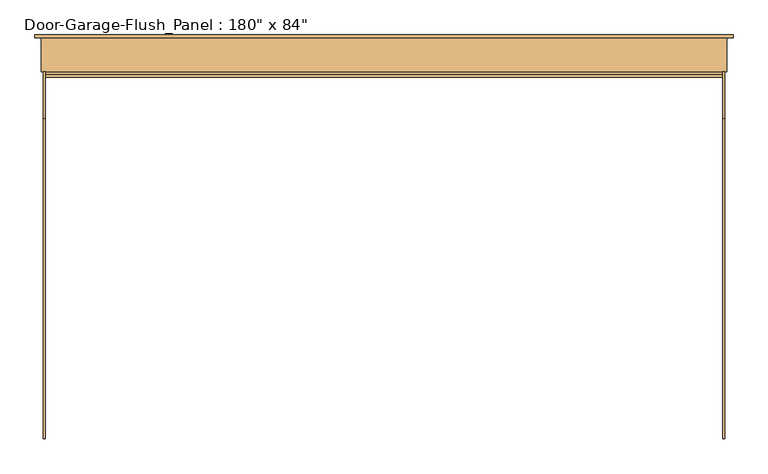
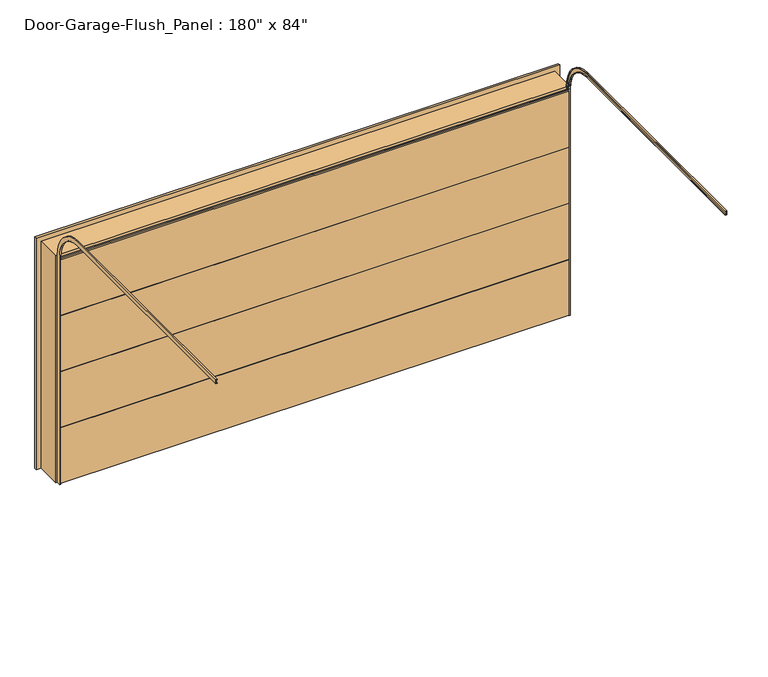
"""IFC4 building model written with IfcOpenShell, lengths in millimetres: door geometry."""

from ifc_helpers import new_model, si_unit, frame, origin, place, context, project, spatial, polyline, circle_curve, outline, extrude, source, transform, mapped, element, save
from ifc_brep_helpers import plane_surface, cylinder_surface, revolved_surface, advanced_brep


def door_0f373a22(model_context):
    return source(origin(), model_context, "Body", "SolidModel", [
        extrude(outline(polyline([(-139.7, 2136.775), (-139.7, 2130.425), (-117.475, 2130.425), (-117.475, 1600.2), (-133.35, 1600.2), (-133.35, 1606.55), (-155.575, 1606.55), (-155.575, 2136.775), (-139.7, 2136.775)])), frame((-2286.0, 0.0, 0.0), z_axis=(1.0, 0.0, 0.0), x_axis=(0.0, 1.0, 0.0)), (0.0, 0.0, 1.0), 4572.0),
        extrude(outline(polyline([(-139.7, 1603.375), (-139.7, 1597.025), (-117.475, 1597.025), (-117.475, 1066.8), (-133.35, 1066.8), (-133.35, 1073.15), (-155.575, 1073.15), (-155.575, 1603.375), (-139.7, 1603.375)])), frame((-2286.0, 0.0, 0.0), z_axis=(1.0, 0.0, 0.0), x_axis=(0.0, 1.0, 0.0)), (0.0, 0.0, 1.0), 4572.0),
        extrude(outline(polyline([(-139.7, 1069.975), (-139.7, 1063.625), (-117.475, 1063.625), (-117.475, 533.4), (-133.35, 533.4), (-133.35, 539.75), (-155.575, 539.75), (-155.575, 1069.975), (-139.7, 1069.975)])), frame((-2286.0, 0.0, 0.0), z_axis=(1.0, 0.0, 0.0), x_axis=(0.0, 1.0, 0.0)), (0.0, 0.0, 1.0), 4572.0),
        extrude(outline(polyline([(-139.7, 536.575), (-139.7, 530.225), (-117.475, 530.225), (-117.475, 0.0), (-133.35, 0.0), (-133.35, 6.35), (-155.575, 6.35), (-155.575, 536.575), (-139.7, 536.575)])), frame((-2286.0, 0.0, 0.0), z_axis=(1.0, 0.0, 0.0), x_axis=(0.0, 1.0, 0.0)), (0.0, 0.0, 1.0), 4572.0),
        advanced_brep(
        [(2298.7, -2593.975, 2438.4), (2298.7, -2593.975, 2476.5), (2286.0, -2593.975, 2476.5), (2286.0, -2593.975, 2473.325), (2295.525, -2593.975, 2473.325), (2295.525, -2593.975, 2441.575), (2286.0, -2593.975, 2441.575), (2286.0, -2593.975, 2438.4), (2298.7, -434.975, 2438.4), (2298.7, -155.575, 2159.0), (2298.7, -155.575, 0.0), (2298.7, -117.475, 0.0), (2298.7, -117.475, 2159.0), (2298.7, -434.975, 2476.5), (2286.0, -434.975, 2476.5), (2286.0, -117.475, 2159.0), (2286.0, -117.475, 0.0), (2286.0, -120.65, 0.0), (2286.0, -120.65, 2159.0), (2286.0, -434.975, 2473.325), (2295.525, -434.975, 2473.325), (2295.525, -120.65, 2159.0), (2295.525, -120.65, 0.0), (2295.525, -152.4, 0.0), (2295.525, -152.4, 2159.0), (2295.525, -434.975, 2441.575), (2286.0, -434.975, 2441.575), (2286.0, -152.4, 2159.0), (2286.0, -152.4, 0.0), (2286.0, -155.575, 0.0), (2286.0, -155.575, 2159.0), (2286.0, -434.975, 2438.4)],
        [
            (0, 1),
            (1, 2),
            (2, 3),
            (3, 4),
            (4, 5),
            (5, 6),
            (6, 7),
            (7, 0),
            (0, 8),
            (8, 9, circle_curve(frame((2298.7, -434.975, 2159.0), z_axis=(-1.0, 0.0, 0.0), x_axis=(0.0, 0.0, 1.0)), 279.4)),
            (9, 10),
            (10, 11),
            (11, 12),
            (12, 13, circle_curve(frame((2298.7, -434.975, 2159.0), z_axis=(1.0, 0.0, 0.0), x_axis=(0.0, 0.0, 1.0)), 317.5)),
            (13, 1),
            (13, 14),
            (14, 2),
            (14, 15, circle_curve(frame((2286.0, -434.975, 2159.0), z_axis=(-1.0, 0.0, 0.0), x_axis=(0.0, 0.0, 1.0)), 317.5)),
            (15, 16),
            (16, 17),
            (17, 18),
            (18, 19, circle_curve(frame((2286.0, -434.975, 2159.0), z_axis=(1.0, 0.0, 0.0), x_axis=(0.0, 0.0, 1.0)), 314.325)),
            (19, 3),
            (19, 20),
            (20, 4),
            (20, 21, circle_curve(frame((2295.525, -434.975, 2159.0), z_axis=(-1.0, 0.0, 0.0), x_axis=(0.0, 0.0, 1.0)), 314.325)),
            (21, 22),
            (22, 23),
            (23, 24),
            (24, 25, circle_curve(frame((2295.525, -434.975, 2159.0), z_axis=(1.0, 0.0, 0.0), x_axis=(0.0, 0.0, 1.0)), 282.575)),
            (25, 5),
            (25, 26),
            (26, 6),
            (26, 27, circle_curve(frame((2286.0, -434.975, 2159.0), z_axis=(-1.0, 0.0, 0.0), x_axis=(0.0, 0.0, 1.0)), 282.575)),
            (27, 28),
            (28, 29),
            (29, 30),
            (30, 31, circle_curve(frame((2286.0, -434.975, 2159.0), z_axis=(1.0, 0.0, 0.0), x_axis=(0.0, 0.0, 1.0)), 279.4)),
            (31, 7),
            (31, 8),
            (12, 15),
            (18, 21),
            (24, 27),
            (30, 9),
            (10, 29),
            (28, 23),
            (22, 17),
            (16, 11),
        ],
        [
            plane_surface(frame((0.0, -2593.975, 2438.4), z_axis=(0.0, -1.0, 0.0), x_axis=(1.0, 0.0, 0.0))),
            plane_surface(frame((2298.7, -2593.975, 2438.4), z_axis=(1.0, 0.0, 0.0), x_axis=(0.0, 1.0, 0.0))),
            plane_surface(frame((2298.7, -2593.975, 2476.5), z_axis=(0.0, 0.0, 1.0), x_axis=(0.0, 1.0, 0.0))),
            plane_surface(frame((2286.0, -2593.975, 2476.5), z_axis=(-1.0, 0.0, 0.0), x_axis=(0.0, 1.0, 0.0))),
            plane_surface(frame((2286.0, -2593.975, 2473.325), z_axis=(0.0, 0.0, -1.0), x_axis=(0.0, 1.0, 0.0))),
            plane_surface(frame((2295.525, -2593.975, 2473.325), z_axis=(-1.0, 0.0, 0.0), x_axis=(0.0, 1.0, 0.0))),
            plane_surface(frame((2295.525, -2593.975, 2441.575), z_axis=(0.0, 0.0, 1.0), x_axis=(0.0, 1.0, 0.0))),
            plane_surface(frame((2286.0, -2593.975, 2441.575), z_axis=(-1.0, 0.0, 0.0), x_axis=(0.0, 1.0, 0.0))),
            plane_surface(frame((2286.0, -2593.975, 2438.4), z_axis=(0.0, 0.0, -1.0), x_axis=(0.0, 1.0, 0.0))),
            cylinder_surface(frame((0.0, -434.975, 2159.0), z_axis=(-1.0, 0.0, 0.0), x_axis=(0.0, 0.0, 1.0)), 317.5),
            revolved_surface(polyline([(2286.0, -434.975, 2473.325), (2295.525, -434.975, 2473.325)]), (0.0, -434.975, 2159.0), (-1.0, 0.0, 0.0)),
            cylinder_surface(frame((0.0, -434.975, 2159.0), z_axis=(-1.0, 0.0, 0.0), x_axis=(0.0, 0.0, 1.0)), 282.575),
            revolved_surface(polyline([(2286.0, -434.975, 2438.4), (2298.7, -434.975, 2438.4)]), (0.0, -434.975, 2159.0), (-1.0, 0.0, 0.0)),
            plane_surface(frame((0.0, -155.575, 0.0), z_axis=(0.0, 0.0, -1.0), x_axis=(1.0, 0.0, 0.0))),
            plane_surface(frame((2298.7, -117.475, 2159.0), z_axis=(0.0, 1.0, 0.0), x_axis=(0.0, 0.0, -1.0))),
            plane_surface(frame((2286.0, -120.65, 2159.0), z_axis=(0.0, -1.0, 0.0), x_axis=(0.0, 0.0, -1.0))),
            plane_surface(frame((2295.525, -152.4, 2159.0), z_axis=(0.0, 1.0, 0.0), x_axis=(0.0, 0.0, -1.0))),
            plane_surface(frame((2286.0, -155.575, 2159.0), z_axis=(0.0, -1.0, 0.0), x_axis=(0.0, 0.0, -1.0))),
        ],
        [
            (0, [[1, 2, 3, 4, 5, 6, 7, 8]]),
            (1, [[-1, 9, 10, 11, 12, 13, 14, 15]]),
            (2, [[-2, -15, 16, 17]]),
            (3, [[-3, -17, 18, 19, 20, 21, 22, 23]]),
            (4, [[-4, -23, 24, 25]]),
            (5, [[-5, -25, 26, 27, 28, 29, 30, 31]]),
            (6, [[-6, -31, 32, 33]]),
            (7, [[-7, -33, 34, 35, 36, 37, 38, 39]]),
            (8, [[-8, -39, 40, -9]]),
            (9, [[-18, -16, -14, 41]]),
            (10, [[-26, -24, -22, 42]]),
            (11, [[-34, -32, -30, 43]]),
            (12, [[-10, -40, -38, 44]]),
            (13, [[45, -36, 46, -28, 47, -20, 48, -12]]),
            (14, [[-41, -13, -48, -19]]),
            (15, [[-42, -21, -47, -27]]),
            (16, [[-43, -29, -46, -35]]),
            (17, [[-44, -37, -45, -11]]),
        ],
    ),
        advanced_brep(
        [(-2298.7, -2593.975, 2438.4), (-2286.0, -2593.975, 2438.4), (-2286.0, -2593.975, 2441.575), (-2295.525, -2593.975, 2441.575), (-2295.525, -2593.975, 2473.325), (-2286.0, -2593.975, 2473.325), (-2286.0, -2593.975, 2476.5), (-2298.7, -2593.975, 2476.5), (-2298.7, -434.975, 2438.4), (-2286.0, -434.975, 2438.4), (-2286.0, -155.575, 2159.0), (-2286.0, -155.575, 0.0), (-2286.0, -152.4, 0.0), (-2286.0, -152.4, 2159.0), (-2286.0, -434.975, 2441.575), (-2295.525, -434.975, 2441.575), (-2295.525, -152.4, 2159.0), (-2295.525, -152.4, 0.0), (-2295.525, -120.65, 0.0), (-2295.525, -120.65, 2159.0), (-2295.525, -434.975, 2473.325), (-2286.0, -434.975, 2473.325), (-2286.0, -120.65, 2159.0), (-2286.0, -120.65, 0.0), (-2286.0, -117.475, 0.0), (-2286.0, -117.475, 2159.0), (-2286.0, -434.975, 2476.5), (-2298.7, -434.975, 2476.5), (-2298.7, -117.475, 2159.0), (-2298.7, -117.475, 0.0), (-2298.7, -155.575, 0.0), (-2298.7, -155.575, 2159.0)],
        [
            (0, 1),
            (1, 2),
            (2, 3),
            (3, 4),
            (4, 5),
            (5, 6),
            (6, 7),
            (7, 0),
            (0, 8),
            (8, 9),
            (9, 1),
            (9, 10, circle_curve(frame((-2286.0, -434.975, 2159.0), z_axis=(-1.0, 0.0, 0.0), x_axis=(0.0, 0.0, 1.0)), 279.4)),
            (10, 11),
            (11, 12),
            (12, 13),
            (13, 14, circle_curve(frame((-2286.0, -434.975, 2159.0), z_axis=(1.0, 0.0, 0.0), x_axis=(0.0, 0.0, 1.0)), 282.575)),
            (14, 2),
            (14, 15),
            (15, 3),
            (15, 16, circle_curve(frame((-2295.525, -434.975, 2159.0), z_axis=(-1.0, 0.0, 0.0), x_axis=(0.0, 0.0, 1.0)), 282.575)),
            (16, 17),
            (17, 18),
            (18, 19),
            (19, 20, circle_curve(frame((-2295.525, -434.975, 2159.0), z_axis=(1.0, 0.0, 0.0), x_axis=(0.0, 0.0, 1.0)), 314.325)),
            (20, 4),
            (20, 21),
            (21, 5),
            (21, 22, circle_curve(frame((-2286.0, -434.975, 2159.0), z_axis=(-1.0, 0.0, 0.0), x_axis=(0.0, 0.0, 1.0)), 314.325)),
            (22, 23),
            (23, 24),
            (24, 25),
            (25, 26, circle_curve(frame((-2286.0, -434.975, 2159.0), z_axis=(1.0, 0.0, 0.0), x_axis=(0.0, 0.0, 1.0)), 317.5)),
            (26, 6),
            (26, 27),
            (27, 7),
            (27, 28, circle_curve(frame((-2298.7, -434.975, 2159.0), z_axis=(-1.0, 0.0, 0.0), x_axis=(0.0, 0.0, 1.0)), 317.5)),
            (28, 29),
            (29, 30),
            (30, 31),
            (31, 8, circle_curve(frame((-2298.7, -434.975, 2159.0), z_axis=(1.0, 0.0, 0.0), x_axis=(0.0, 0.0, 1.0)), 279.4)),
            (31, 10),
            (13, 16),
            (19, 22),
            (25, 28),
            (29, 24),
            (23, 18),
            (17, 12),
            (11, 30),
        ],
        [
            plane_surface(frame((0.0, -2593.975, 2438.4), z_axis=(0.0, -1.0, 0.0), x_axis=(1.0, 0.0, 0.0))),
            plane_surface(frame((-2298.7, -2593.975, 2438.4), z_axis=(0.0, 0.0, -1.0), x_axis=(0.0, 1.0, 0.0))),
            plane_surface(frame((-2286.0, -2593.975, 2438.4), z_axis=(1.0, 0.0, 0.0), x_axis=(0.0, 1.0, 0.0))),
            plane_surface(frame((-2286.0, -2593.975, 2441.575), z_axis=(0.0, 0.0, 1.0), x_axis=(0.0, 1.0, 0.0))),
            plane_surface(frame((-2295.525, -2593.975, 2441.575), z_axis=(1.0, 0.0, 0.0), x_axis=(0.0, 1.0, 0.0))),
            plane_surface(frame((-2295.525, -2593.975, 2473.325), z_axis=(0.0, 0.0, -1.0), x_axis=(0.0, 1.0, 0.0))),
            plane_surface(frame((-2286.0, -2593.975, 2473.325), z_axis=(1.0, 0.0, 0.0), x_axis=(0.0, 1.0, 0.0))),
            plane_surface(frame((-2286.0, -2593.975, 2476.5), z_axis=(0.0, 0.0, 1.0), x_axis=(0.0, 1.0, 0.0))),
            plane_surface(frame((-2298.7, -2593.975, 2476.5), z_axis=(-1.0, 0.0, 0.0), x_axis=(0.0, 1.0, 0.0))),
            revolved_surface(polyline([(-2298.7, -434.975, 2438.4), (-2286.0, -434.975, 2438.4)]), (0.0, -434.975, 2159.0), (-1.0, 0.0, 0.0)),
            cylinder_surface(frame((0.0, -434.975, 2159.0), z_axis=(-1.0, 0.0, 0.0), x_axis=(0.0, 0.0, 1.0)), 282.575),
            revolved_surface(polyline([(-2295.525, -434.975, 2473.325), (-2286.0, -434.975, 2473.325)]), (0.0, -434.975, 2159.0), (-1.0, 0.0, 0.0)),
            cylinder_surface(frame((0.0, -434.975, 2159.0), z_axis=(-1.0, 0.0, 0.0), x_axis=(0.0, 0.0, 1.0)), 317.5),
            plane_surface(frame((0.0, -155.575, 0.0), z_axis=(0.0, 0.0, -1.0), x_axis=(1.0, 0.0, 0.0))),
            plane_surface(frame((-2298.7, -155.575, 2159.0), z_axis=(0.0, -1.0, 0.0), x_axis=(0.0, 0.0, -1.0))),
            plane_surface(frame((-2286.0, -152.4, 2159.0), z_axis=(0.0, 1.0, 0.0), x_axis=(0.0, 0.0, -1.0))),
            plane_surface(frame((-2295.525, -120.65, 2159.0), z_axis=(0.0, -1.0, 0.0), x_axis=(0.0, 0.0, -1.0))),
            plane_surface(frame((-2286.0, -117.475, 2159.0), z_axis=(0.0, 1.0, 0.0), x_axis=(0.0, 0.0, -1.0))),
        ],
        [
            (0, [[1, 2, 3, 4, 5, 6, 7, 8]]),
            (1, [[-1, 9, 10, 11]]),
            (2, [[-2, -11, 12, 13, 14, 15, 16, 17]]),
            (3, [[-3, -17, 18, 19]]),
            (4, [[-4, -19, 20, 21, 22, 23, 24, 25]]),
            (5, [[-5, -25, 26, 27]]),
            (6, [[-6, -27, 28, 29, 30, 31, 32, 33]]),
            (7, [[-7, -33, 34, 35]]),
            (8, [[-8, -35, 36, 37, 38, 39, 40, -9]]),
            (9, [[-12, -10, -40, 41]]),
            (10, [[-20, -18, -16, 42]]),
            (11, [[-28, -26, -24, 43]]),
            (12, [[-36, -34, -32, 44]]),
            (13, [[-38, 45, -30, 46, -22, 47, -14, 48]]),
            (14, [[-41, -39, -48, -13]]),
            (15, [[-42, -15, -47, -21]]),
            (16, [[-43, -23, -46, -29]]),
            (17, [[-44, -31, -45, -37]]),
        ],
    ),
        extrude(outline(polyline([(0.0, 2286.0), (0.0, 2311.4), (2159.0, 2311.4), (2159.0, -2311.4), (0.0, -2311.4), (0.0, -2286.0), (2133.6, -2286.0), (2133.6, 2286.0), (0.0, 2286.0)])), frame((0.0, -117.475, 0.0), z_axis=(0.0, 1.0, 0.0), x_axis=(0.0, 0.0, 1.0)), (0.0, 0.0, 1.0), 228.6),
        extrude(outline(polyline([(0.0, 2292.35), (0.0, 2355.85), (2203.45, 2355.85), (2203.45, -2355.85), (0.0, -2355.85), (0.0, -2292.35), (2139.95, -2292.35), (2139.95, 2292.35), (0.0, 2292.35)])), frame((0.0, 111.125, 0.0), z_axis=(0.0, 1.0, 0.0), x_axis=(0.0, 0.0, 1.0)), (0.0, 0.0, 1.0), 19.05),
    ])


if __name__ == "__main__":
    model = new_model("IFC4")
    model_context = context("Model", 3, world=origin())
    ifc_project = project(units=[si_unit("LENGTHUNIT", "METRE", prefix="MILLI")], contexts=[model_context])
    site = spatial("IfcSite", under=ifc_project)
    building = spatial("IfcBuilding", under=site)
    placement = place(None, origin())
    door_shape = door_0f373a22(model_context)
    element("IfcDoor", 1, ObjectType="Door-Garage-Flush_Panel : 180\" x 84\"", at=placement, inside=building, context=model_context, shape_type="MappedRepresentation", body=[
        mapped(door_shape, transform((0.0, 0.0, 0.0), x_axis=(1.0, 0.0, 0.0), y_axis=(0.0, 1.0, 0.0), z_axis=(0.0, 0.0, 1.0))),
    ])
    save(model, "model.ifc")

# Revit data of these elements
# Type "Door-Garage-Flush_Panel : 180\" x 84\""
#   Type Mark = "12"
#   Assembly Code = "B2030400"
#   Analytic Construction = "Wooden"
#   Thickness = 0' - 1 1/2"
#   Thermal Resistance (R) = 2.5876 (h·ft²·°F)/BTU
#   Rough Width = 15' - 2"
#   Rough Height = 7' - 1"
#   Panel Height = 1' - 9"
#   Height = 7' - 0"
#   Width = 15' - 0"
#   Heat Transfer Coefficient (U) = 0.3865 BTU/(h·ft²·°F)
#   Function = 1
#   Exterior Trim [instance default] = yes
#   Trim Material = Cherry
#   Panel Material = Cherry
#   Frame Material = Cherry
#   Visual Light Transmittance = 0
#   Solar Heat Gain Coefficient = 0
#   Wall Closure = (empty or 0)
# Element 1 (IfcDoor, "Door-Garage-Flush_Panel : 180\" x 84\"")
#   Materials on its faces: "Cherry"
# Materials
#   "Cherry": class "Wood", colour RGB 226 177 128, transparency 0, Description = "Prunus Serotina", Cost = 0
